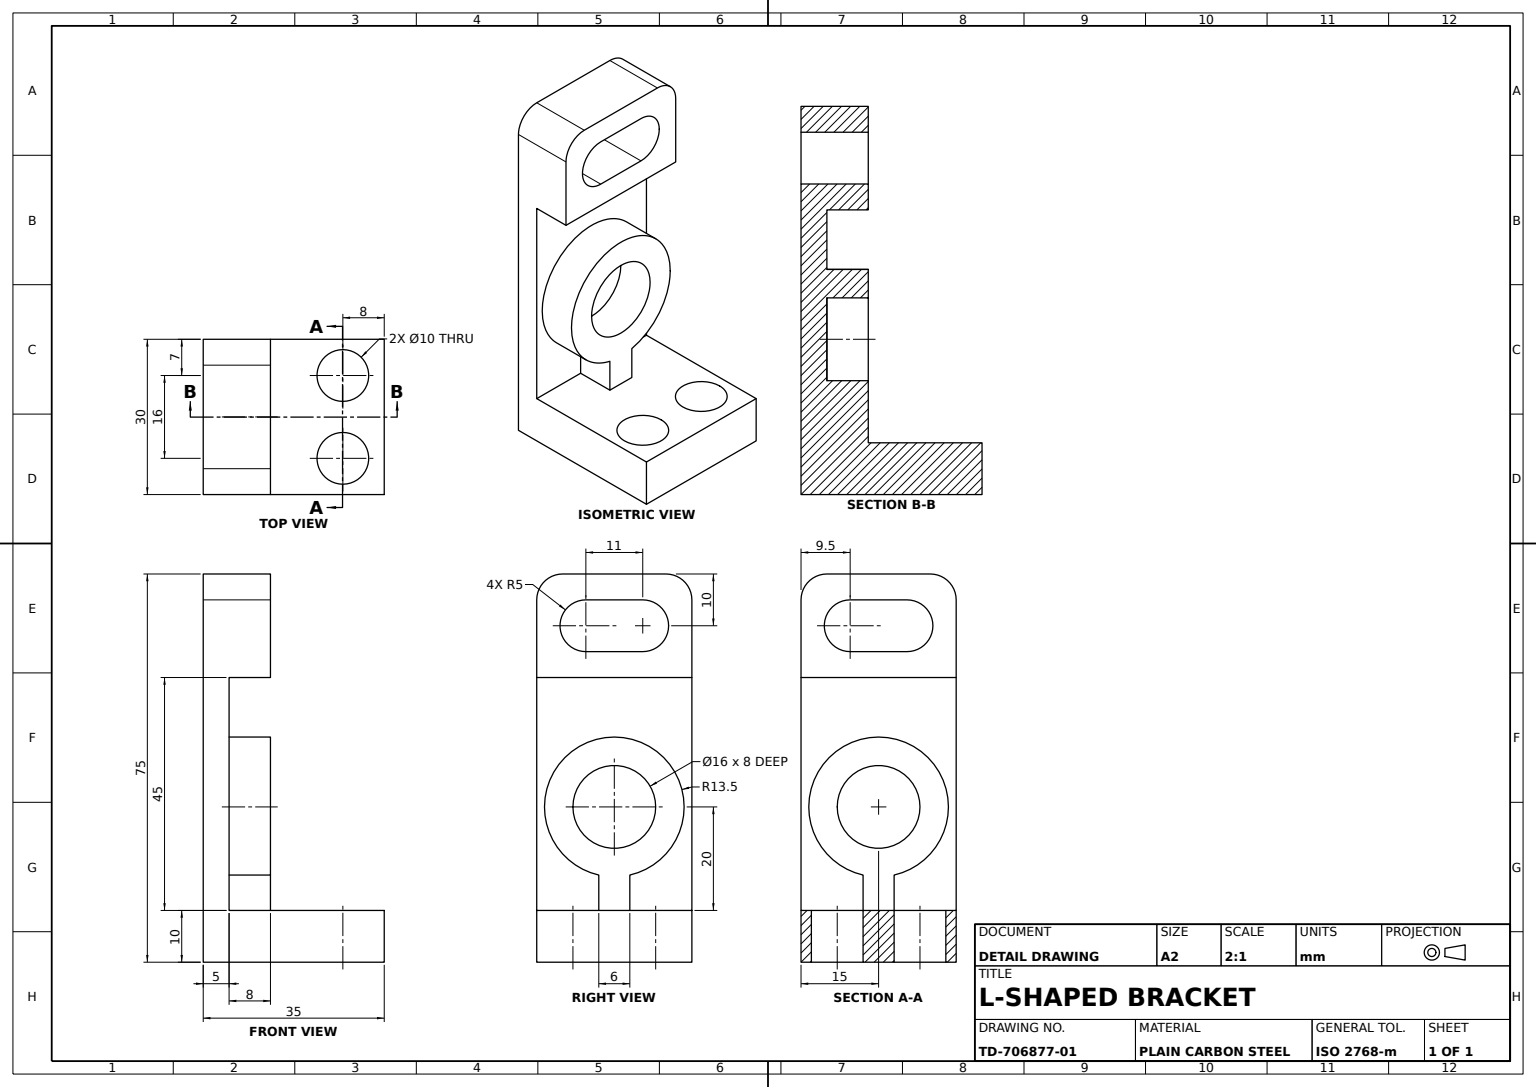
SolidWorks part; units mm, degrees
material "Plain Carbon Steel"
ref_plane "Front Plane" through (0, 0, 0) normal (0, 0, 1) x (1, 0, 0)
ref_plane "Top Plane" through (0, 0, 0) normal (0, 1, 0) x (1, 0, 0)
ref_plane "Right Plane" through (0, 0, 0) normal (1, 0, 0) x (0, 0, -1)
sketch "Base Plate Sketch" plane through (0, 0, 0) normal (0, 0, 1) x (1, 0, 0)
  line L1 (0, 0) -> (35, 0)
  line L2 (0, 0) -> (0, 10)
  line L3 (0, 10) -> (35, 10)
  line L4 (35, 0) -> (35, 10)
  dimension "D1" = 35
  dimension "D2" = 10
extrude "Base Plate" add sketch "Base Plate Sketch" against normal blind 30
sketch "Upright Wall Sketch" plane through (0, 0, 0) normal (0, 0, 1) x (1, 0, 0)
  line L1 (0, 10) -> (5, 10)
  line L2 (0, 10) -> (0, 55)
  line L3 (0, 55) -> (5, 55)
  line L4 (5, 10) -> (5, 55)
  dimension "D1" = 45
  dimension "D2" = 5
extrude "Upright Wall" add sketch "Upright Wall Sketch" against normal blind 30
sketch "Mounting Holes Sketch" plane through (0, 10, 0) normal (0, 1, 0) x (1, 0, 0)
  line L0 (35, 30) -> (35, 0) construction
  line L1 (35, 0) -> (5, 0) construction
  line L2 (35, 30) -> (5, 30) construction
  circle A0 centre (27, 23) radius 5
  circle A1 centre (27, 7) radius 5
  dimension "D4" = 10
  dimension "D1" = 8
  dimension "D2" = 7
  dimension "D3" = 7
extrude "Mounting Holes 2x" cut sketch "Mounting Holes Sketch" against normal blind 30
sketch "Top Lug Sketch" plane through (5, 0, 0) normal (1, 0, 0) x (0, 0, -1)
  line L1 (0, 55) -> (30, 55)
  line L2 (0, 55) -> (0, 70)
  line L3 (5, 75) -> (25, 75)
  line L4 (30, 55) -> (30, 70)
  arc A0 (25, 75) -> (30, 70) centre (25, 70) cw
  arc A1 (0, 70) -> (5, 75) centre (5, 70) cw
  point P9 (0, 75)
  dimension "D3" = 5
  dimension "D1" = 20
  dimension "D2" = 30
extrude "Top Lug" add sketch "Top Lug Sketch" along normal blind 8 and the other way blind 5
sketch "Lug Slot Sketch" plane through (13, 0, 0) normal (1, 0, 0) x (0, 0, -1)
  line L0 (0, 65) -> (32.2108, 65) construction
  line L1 (0, 70) -> (0, 55) construction
  line L2 (0, 55) -> (30, 55) construction
  line L3 (15, 55) -> (15, 75) construction
  line L4 (30, 55) -> (0, 55) construction
  line L5 (9.5, 65) -> (20.5, 65) construction
  line L6 (9.5, 70) -> (20.5, 70)
  line L7 (9.5, 60) -> (20.5, 60)
  arc A0 (9.5, 70) -> (9.5, 60) centre (9.5, 65) ccw
  arc A1 (20.5, 60) -> (20.5, 70) centre (20.5, 65) ccw
  point P12 (15, 65)
  dimension "D1" = 10
  dimension "D2" = 11
  dimension "D3" = 10
extrude "Lug Slot" cut sketch "Lug Slot Sketch" against normal through all
sketch "Ring Boss Sketch" plane through (5, 0, 0) normal (1, 0, 0) x (0, 0, -1)
  line L0 (15, 10) -> (15, 43.5566) construction
  line L1 (30, 10) -> (0, 10) construction
  line L2 (5.2418, 30) -> (25.9616, 30) construction
  line L3 (0, 10) -> (0, 55) construction
  line L4 (12, 16.8376) -> (12, 10)
  line L5 (18, 16.8376) -> (18, 10)
  line L6 (12, 10) -> (18, 10)
  circle A0 centre (15, 30) radius 8
  arc A1 (18, 16.8376) -> (12, 16.8376) centre (15, 30) ccw
  point P9 (15, 18.374)
  point P10 (12, 18.374)
  point P12 (18, 18.374)
  dimension "D2" = 16
  dimension "D3" = 27
  dimension "D1" = 20
  dimension "D4" = 12
extrude "Ring Boss" add sketch "Ring Boss Sketch" along normal blind 8
